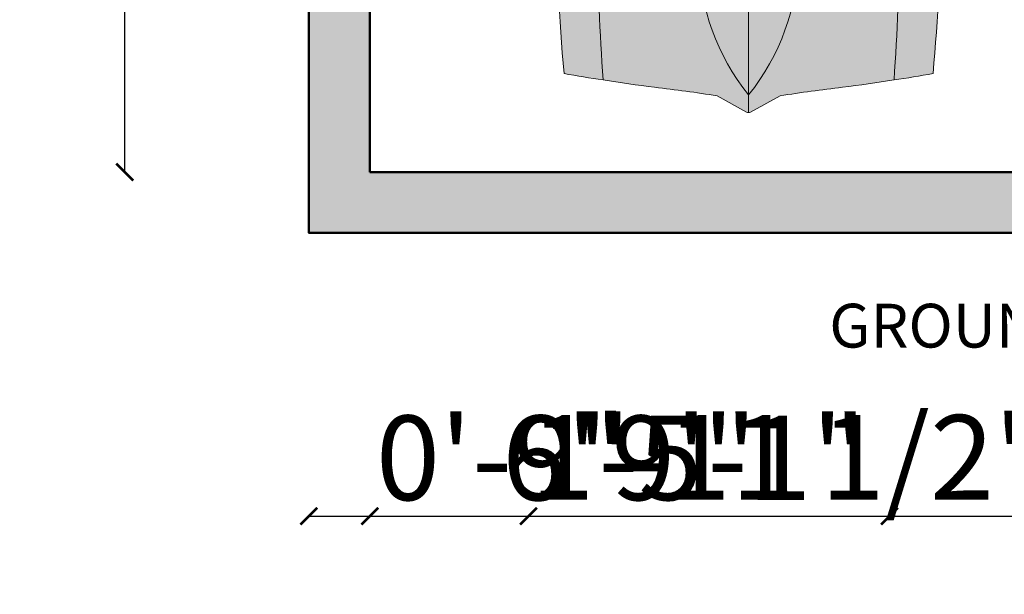
# Model space of a CAD drawing. Units: inches. Extents: x 2419 to 2878, y 1068 to 1713.
# Tile 1 of 20: x 2429 to 2574, y 1068 to 1153. Entities that reach past the tile are written whole.
import ezdxf

# ---------------------------------------------------------------- set-up
doc = ezdxf.new("R2010")
doc.units = ezdxf.units.IN
for name, color, linetype, lineweight in [('A-ANNO-DIMS', 2, 'Continuous', 18), ('A-ANNO-TEXT', 7, 'Continuous', 25), ('A-FLOR-PRKG', 8, 'Continuous', 13), ('A-FLOR-PRKG-PATT', 1, 'Continuous', 13), ('A-WALL', 7, 'Continuous', 50)]:
    doc.layers.add(name, color=color, linetype=linetype, lineweight=lineweight)
doc.layers.add('A-WALL-PATT', color=18, linetype='Continuous', lineweight=13, true_color=0x000000)
doc.styles.get("Standard").update_dxf_attribs({"font": 'arial.ttf'})
doc.dimstyles.new('ISO-25', dxfattribs={"dimtxt": 12.5, "dimasz": 2.5, "dimexe": 1.25, "dimexo": 0.625, "dimtad": 1, "dimdec": 0, "dimlunit": 4, "dimtxsty": 'Standard', "dimblk": 'ARCHTICK', "dimcen": 2.5, "dimse1": 1, "dimse2": 1, "dimclrd": 4, "dimadec": 0, "dimazin": 0, "dimtfac": 1, "dimtdec": 0, "dimtmove": 0, "dimatfit": 3, "dimfxl": 1, "dimarcsym": 0})

# ---------------------------------------------------------------- blocks, each defined once
blk = doc.blocks.new('*U7')
for p, q in [((46.55368679439944, 38.88847654282876), (22.35054758993934, 38.88847654282876)), ((136.6978032355602, 38.88847654282876), (160.90094244002, 38.88847654282867)), ((21.10406751471477, 37.40863046792069), (21.10406751471477, 36.83230215753705)), ((47.80016686962392, 37.39011648242055), (47.80016686962392, 37.40863046792069)), ((135.4513231603356, 37.07354110333037), (135.4513231603356, 37.40863046792069)), ((162.1474225152445, 37.40863046792049), (162.1474225152445, 36.77402019194128)), ((87.98532186932616, 31.87120872459877), (74.75900729854769, 35.92175679182955)), ((134.313356548143, 35.6043097713567), (119.2882629232503, 31.77757799177584)), ((186.4728846989705, -33.49860931502491), (186.4728846989718, 33.49860931502465)), ((188.3990091454065, -32.75868627757393), (188.3990091454077, 32.75868627757058)), ((70.0302824853563, 31.53613089391356), (86.40615155322342, 29.35124891408057)), ((138.4228833961707, 29.35124891408074), (157.2465674415997, 29.35124891408074)), ((186.4728846989718, 29.35124891408083), (167.0083537481071, 29.35124891408083)), ((164.515393597658, 26.39155676426461), (164.5153935976578, -26.39155676426503)), ((32.26591480791686, 11.62530558863241), (36.12873726252356, 17.16961494239206)), ((36.12873726252356, 17.16961494239206), (50.93891189819171, 17.16961494239206)), ((32.12291633764599, 9.505833383620029), (32.12291633764599, 11.15369945057711)), ((58.9167604809788, -10.77488335095668), (58.9167604809788, 10.77488335095617)), ((66.55009204259746, -10.5288681329018), (66.55009204259746, 10.52886813290129)), ((186.4728846989718, -10.5288681329018), (186.4728846989718, 10.52886813290129)), ((29.77279020470884, 9.505833383620029), (51.68362801571248, 9.505833383620029)), ((82.73706193978568, 8.496039918672748), (82.73706193978568, -8.49603991867258)), ((3.266462181856987, 6.128290093440767), (0.1022408397004821, 0.4060708604429806)), ((-4.43e-14, -2.558e-13), (51.68362801571248, -2.558e-13)), ((0.1022408397004821, -0.4060708604432933), (3.266462181856987, -6.128290093441194)), ((29.77279020470884, -9.50583338362054), (51.68362801571248, -9.50583338362054)), ((32.12291633764599, -9.50583338362054), (32.12291633764599, -11.15369945057762)), ((32.26591480791686, -11.62530558863292), (36.12873726252356, -17.16961494239257)), ((36.12873726252356, -17.16961494239257), (50.93891189819171, -17.16961494239257)), ((86.40615155322318, -29.35124891408145), (70.03028248535594, -31.53613089391442)), ((157.2465674415997, -29.35124891408117), (138.4228833961707, -29.35124891408126)), ((167.008353748107, -29.35124891408126), (186.4728846989707, -29.35124891408108)), ((87.98532186932607, -31.87120872459903), (74.7590072985476, -35.92175679182964)), ((134.3133565481428, -35.60430977135721), (119.2882629232503, -31.77757799177618)), ((21.10406751471477, -37.4086304679212), (21.10406751471477, -36.83230215753756)), ((47.80016686962392, -37.39011648242107), (47.80016686962392, -37.4086304679212)), ((135.4513231603355, -37.07354110333088), (135.4513231603355, -37.4086304679212)), ((162.1474225152445, -37.408630467921), (162.1474225152445, -36.77402019194179)), ((46.55368679439944, -38.88847654282927), (22.35054758993934, -38.88847654282927)), ((136.6978032355602, -38.88847654282927), (160.9009424400199, -38.88847654282918))]:
    blk.add_line(p, q)
for centre, major_axis, ratio, start_param, end_param in [((22.35054758993934, 37.40863046792072), (2.08e-14, -1.479846074908118), 0.842303869543976, 3.141592653589776, 4.712388980384677), ((46.55368679439944, 37.40863046792072), (2.2e-14, 1.479846074908118), 0.8423038695439758, -1.570796326794884, 1.73e-14), ((136.6978032355602, 37.40863046792072), (2.357e-13, -1.479846074908118), 0.842303869543976, 3.141592653589603, 4.712388980384554), ((160.90094244002, 37.40863046792052), (5.59e-14, 1.479846074908118), 0.842303869543976, -1.570796326794865, 4.44e-14), ((41.19115208863305, -490.8631038926156), (1.294e-13, 528.2339998381949), 0.8423038695439741, 0.0028100083536837, 0.0755983031096952), ((64.48199294511879, -10555.61767587835), (1.907644e-10, 10593.02630634627), 0.842303869543847, -0.0133969486112073, 0.0027970409639888), ((180.6280394947615, 35.8381667808375), (7.4e-14, 2.219769112362114), 0.8423038695439693, -0.0130174256259048, 1.249894140392862), ((64.48199294754608, -10556.35759891604), (1.349839377e-06, 10595.3130398087), 0.8423038681351469, -0.0133969484821159, -0.0130174254969711), ((183.9799245485226, 33.49860931502124), (3e-16, -2.959692149816168), 0.8423038695439952, 1.570796326796048, 3.128195704978389), ((183.9799245485216, 32.75868627756583), (8.56e-14, -5.246425615115243), 0.8423038695439737, 1.570796326795794, 3.128195704978164), ((266.0300214172791, -27.52442688366631), (1.966072e-10, 313.3077612809058), 0.8423038695435284, 1.367075990158062, 1.391760499156098), ((64.4819929449925, -10555.61767590795), (1.9177683e-09, -10591.54646030096), 0.8423038695482963, 3.133765086725325, 3.140440689641252), ((135.2911776514449, 5.387441675478555), (2.2715e-12, 81.77258453065997), 0.8423038695439563, 1.245306111696802, 1.507880129813836), ((95.78879860270445, -3666.353346297651), (1.949864e-10, -3698.236159209632), 0.8423038695446962, 3.134048706297306, 3.14409775411291), ((37.47375371777758, -593.9621830607928), (6.21e-14, -623.32820996736), 0.8423038695439826, 3.09604606856106, 3.200911180495224), ((134.4003789125686, 5.387441675477674), (4.276e-13, -89.7774543484738), 0.84230386954398, 4.44948196380473, 4.652344057257214), ((149.595361812917, 2.799442537139299), (8.561e-13, -79.57966406425402), 0.842303869543983, 4.372215489277867, 4.640744122441986), ((17.08207736189386, -1.421e-13), (6.87e-14, 147.0179238898305), 0.8423038695439764, 4.511394369635731, 4.913383591133647), ((35.90576140732288, -1.421e-13), (6.87e-14, 147.0179238898305), 0.8423038695439764, 4.511394369635731, 4.913383591133647), ((167.0083537481071, 26.39155676426464), (1.394e-13, 2.959692149816236), 0.842303869543976, 5.55e-14, 1.57079632679492), ((259.1750197310735, -27.52442688366614), (1.506617e-10, -305.3028914627677), 0.8423038695443789, 4.528606069860317, 4.561837674556238), ((-204.4946649195746, 52.39684969293512), (4.12053e-11, -250.9602162198571), 0.8423038695441164, 1.385369446298923, 1.434372047871027), ((13.03653510440275, 17.00972444508943), (1.2303e-12, 27.41599049210566), 0.8423038695439277, 4.435146050259648, 4.718221029521873), ((14.20086229321332, 17.00972444508943), (1.2303e-12, 27.41599049210566), 0.8423038695439277, 4.435146050259648, 4.718221029521873), ((50.7902773840875, 13.33772416300607), (6.340077547122382, -0.356608581037027), 0.6038335755719145, -1.39555193967809, 1.581314658479915), ((32.74615637525823, 11.15369945057713), (1.313e-13, 0.7399230374541176), 0.8423038695439091, 0.8797135699495516, 1.570796326795045), ((29.77279020470884, -46.66302566589627), (5.12e-14, 56.16885904951626), 0.842303869543976, 7e-16, 0.5903187773915901), ((0.6232400376122422, -1.421e-13), (1e-16, -0.7399230374541245), 0.842303869543842, 4.131459131953847, 5.293318828815531), ((29.77279020470884, 46.66302566589578), (4.004e-13, 56.16885904951626), 0.8423038695439734, 2.55127387619821, 3.141592653589801), ((-204.4946649195746, -52.39684969293552), (4.02945e-11, 250.9602162198562), 0.8423038695441192, -1.43437204787103, -1.385369446298926), ((13.03653510440275, -17.00972444508983), (1.2568e-12, -27.41599049210552), 0.8423038695439318, 1.564964277657711, 1.848039256919935), ((14.20086229321332, -17.00972444508983), (1.2568e-12, -27.41599049210552), 0.8423038695439318, 1.564964277657711, 1.848039256919935), ((149.5953618129329, -2.799442537137565), (4.0897e-12, -79.57966406427697), 0.8423038695439419, -1.499151468852248, -1.230622835688196), ((32.74615637525823, -11.1536994505777), (1.3e-13, -0.7399230374541176), 0.8423038695439093, 4.712388980384541, 5.403471737230034), ((134.4003789125684, -5.387441675478584), (4.2949e-12, -89.77745434847827), 0.8423038695439354, -1.510751403667474, -1.307889310215002), ((135.2911776514465, -5.387441675480715), (3.2038e-12, -81.77258453066244), 0.8423038695439492, -1.50788012981387, -1.245306111696839), ((259.1750197310694, 27.52442688365929), (1.08535e-11, 305.3028914629043), 0.8423038695439974, 1.721347632622872, 1.754579237318777), ((167.008353748107, -26.39155676426503), (1.02e-14, -2.959692149816192), 0.8423038695439885, 4.712388980384686, 6.283185307179581), ((266.0300214172791, 27.52442688366566), (8.75241e-11, 313.3077612806533), 0.8423038695441819, 1.749832154434603, 1.774516663432659), ((37.47375371777847, 593.9621830607904), (1.1693e-12, -623.3282099673584), 0.8423038695439528, -0.0593185269054384, 0.0455465850287298), ((95.78879860271888, 3666.35334629765), (1.637818e-10, -3698.236159209629), 0.8423038695447546, -0.0025051005232382, 0.007543947292366), ((183.9799245485216, -33.4986093150211), (9.3e-15, 2.959692149816141), 0.8423038695439732, 3.154989602201626, 4.71238898038339), ((183.9799245485177, -32.7586862775633), (2.428e-13, -5.246425615118353), 0.8423038695439808, 0.0133969486110846, 1.570796326792831), ((41.19115208863322, 490.8631038926152), (1.37757e-11, -528.2339998381949), 0.8423038695440652, -0.0755983031097181, -0.0028100083537155), ((64.48199294503607, 10555.61767590793), (1.6049794e-09, -10591.54646030094), 0.8423038695397146, 0.0011519639481523, 0.0078275668641468), ((22.35054758993934, -37.40863046792117), (2.2e-14, 1.479846074908118), 0.8423038695439758, 1.570796326794908, 3.14159265358981), ((64.48199294495228, 10555.61767590795), (6.117947e-10, 10593.02630637587), 0.8423038695458146, 3.138795612625926, 3.154989602201039), ((46.55368679439944, -37.40863046792117), (2.08e-14, -1.479846074908118), 0.842303869543976, -1.69e-14, 1.570796326794884), ((136.6978032355602, -37.40863046792109), (1.56e-14, -1.479846074908162), 0.8423038695440105, -1.570796326794875, -1.27e-14), ((160.9009424400199, -37.408630467921), (1.969e-13, 1.479846074908162), 0.8423038695440109, 3.141592653589951, 4.712388980384771), ((180.6280394947581, -35.83816678083949), (2.274e-13, -2.219769112363032), 0.8423038695439803, -1.249894138785958, 0.0130174256254374), ((64.48199294197605, 10556.3575989598), (9.365289701e-07, 10595.31303985772), 0.8423038705260315, 3.154610079306566, 3.154989602290631)]:
    blk.add_ellipse(centre, major_axis=major_axis, ratio=ratio, start_param=start_param, end_param=end_param)
at = {"extrusion": (0, 0, -1)}
blk.add_ellipse((50.7902773840875, -13.33772416300655), major_axis=(6.340077547122382, 0.3566085810370246), ratio=0.6038335755719145, start_param=-1.39555193967809, end_param=1.581314658479915, dxfattribs=at)
blk = doc.blocks.new('_ArchTick')
at = {"color": 0, "linetype": 'ByBlock', "const_width": 0.15}
blk.add_lwpolyline([(-0.5, -0.5), (0.5, 0.5)], dxfattribs=at)
blk = doc.blocks.new('*D38')
at = {"layer": 'A-ANNO-DIMS', "color": 4, "lineweight": -2, "transparency": 16777216}
for p, q in [((2444.314464000002, 1165.602617), (2444.314464000002, 1212.505754789905)), ((2444.314464000002, 1130.812987), (2444.314464000002, 1165.602617))]:
    blk.add_line(p, q, dxfattribs=at)
at = {"layer": 'Defpoints', "color": 0, "transparency": 16777216}
for p in [(2444.314464000002, 1165.602617), (2656.740829000001, 1165.602617), (2656.740829000001, 1130.812987)]:
    blk.add_point(p, dxfattribs=at)
at = {"layer": 'A-ANNO-DIMS', "color": 4, "lineweight": -2, "transparency": 16777216, "xscale": 2.5, "yscale": 2.5, "zscale": 2.5}
for p, rotation in [((2444.314464000002, 1165.602617), 90), ((2444.314464000002, 1130.812987), 270)]:
    blk.add_blockref('_ArchTick', p, dxfattribs=dict(at, rotation=rotation))
at = {"layer": 'A-ANNO-DIMS', "color": 0, "transparency": 16777216, "insert": (2437.413884190998, 1190.304185894951), "char_height": 12.5, "attachment_point": 5, "rotation": 90}
blk.add_mtext('2\'-11"', dxfattribs=at)
blk = doc.blocks.new('*D41')
at = {"layer": 'A-ANNO-DIMS', "color": 4, "lineweight": -2, "transparency": 16777216}
for p, q in [((2471.514464, 1079.924615), (2480.514464, 1079.924615)), ((2480.514464, 1079.924615), (2517.492635896316, 1079.924615))]:
    blk.add_line(p, q, dxfattribs=at)
at = {"layer": 'Defpoints', "color": 0, "transparency": 16777216}
for p in [(2480.514464, 1130.812987), (2471.514464, 1121.812987), (2480.514464, 1079.924615)]:
    blk.add_point(p, dxfattribs=at)
at = {"layer": 'A-ANNO-DIMS', "color": 4, "lineweight": -2, "transparency": 16777216, "xscale": 2.5, "yscale": 2.5, "zscale": 2.5, "rotation": 180}
blk.add_blockref('_ArchTick', (2471.514464, 1079.924615), dxfattribs=at)
at = {"layer": 'A-ANNO-DIMS', "color": 4, "lineweight": -2, "transparency": 16777216, "xscale": 2.5, "yscale": 2.5, "zscale": 2.5}
blk.add_blockref('_ArchTick', (2480.514464, 1079.924615), dxfattribs=at)
at = {"layer": 'A-ANNO-DIMS', "color": 0, "transparency": 16777216, "insert": (2500.253549948158, 1086.931777346521), "char_height": 12.5, "attachment_point": 5}
blk.add_mtext('0\'-9"', dxfattribs=at)
blk = doc.blocks.new('*D43')
at = {"layer": 'A-ANNO-DIMS', "color": 4, "lineweight": -2, "transparency": 16777216}
blk.add_line((2480.514464, 1079.924615), (2557.299401, 1079.924615), dxfattribs=at)
at = {"layer": 'Defpoints', "color": 0, "transparency": 16777216}
for p in [(2480.514464, 1408.812987), (2557.299401, 1408.812987), (2557.299401, 1079.924615)]:
    blk.add_point(p, dxfattribs=at)
at = {"layer": 'A-ANNO-DIMS', "color": 4, "lineweight": -2, "transparency": 16777216, "xscale": 2.5, "yscale": 2.5, "zscale": 2.5, "rotation": 180}
blk.add_blockref('_ArchTick', (2480.514464, 1079.924615), dxfattribs=at)
at = {"layer": 'A-ANNO-DIMS', "color": 4, "lineweight": -2, "transparency": 16777216, "xscale": 2.5, "yscale": 2.5, "zscale": 2.5}
blk.add_blockref('_ArchTick', (2557.299401, 1079.924615), dxfattribs=at)
at = {"layer": 'A-ANNO-DIMS', "color": 0, "transparency": 16777216, "insert": (2518.9069325, 1086.931777346521), "char_height": 12.5, "attachment_point": 5}
blk.add_mtext('6\'-5"', dxfattribs=at)
blk = doc.blocks.new('*D44')
at = {"layer": 'A-ANNO-DIMS', "color": 4, "lineweight": -2, "transparency": 16777216}
for p, q in [((2557.299401, 1079.924615), (2585.817994, 1079.924615)), ((2585.817994, 1079.924615), (2652.136206824011, 1079.924615))]:
    blk.add_line(p, q, dxfattribs=at)
at = {"layer": 'Defpoints', "color": 0, "transparency": 16777216}
for p in [(2557.299401, 1408.812987), (2585.817994, 1408.812987), (2585.817994, 1079.924615)]:
    blk.add_point(p, dxfattribs=at)
at = {"layer": 'A-ANNO-DIMS', "color": 4, "lineweight": -2, "transparency": 16777216, "xscale": 2.5, "yscale": 2.5, "zscale": 2.5, "rotation": 180}
blk.add_blockref('_ArchTick', (2557.299401, 1079.924615), dxfattribs=at)
at = {"layer": 'A-ANNO-DIMS', "color": 4, "lineweight": -2, "transparency": 16777216, "xscale": 2.5, "yscale": 2.5, "zscale": 2.5}
blk.add_blockref('_ArchTick', (2585.817994, 1079.924615), dxfattribs=at)
at = {"layer": 'A-ANNO-DIMS', "color": 0, "transparency": 16777216, "insert": (2620.227100412006, 1087.012780075034), "char_height": 12.5, "attachment_point": 5}
blk.add_mtext('2\'-4 1/2"', dxfattribs=at)
blk = doc.blocks.new('*D54')
at = {"layer": 'A-ANNO-DIMS', "color": 4, "lineweight": -2, "transparency": 16777216}
blk.add_line((2444.314464000002, 1130.812987), (2444.314464000002, 1293.812987), dxfattribs=at)
at = {"layer": 'Defpoints', "color": 0, "transparency": 16777216}
for p in [(2444.314464000002, 1293.812987), (2480.514464000001, 1293.812987), (2480.514464000001, 1130.812987)]:
    blk.add_point(p, dxfattribs=at)
at = {"layer": 'A-ANNO-DIMS', "color": 4, "lineweight": -2, "transparency": 16777216, "xscale": 2.5, "yscale": 2.5, "zscale": 2.5}
for p, rotation in [((2444.314464000002, 1293.812987), 90), ((2444.314464000002, 1130.812987), 270)]:
    blk.add_blockref('_ArchTick', p, dxfattribs=dict(at, rotation=rotation))
at = {"layer": 'A-ANNO-DIMS', "color": 0, "transparency": 16777216, "insert": (2437.30303835198, 1212.312987), "char_height": 12.5, "attachment_point": 5, "rotation": 90}
blk.add_mtext('13\'-7"', dxfattribs=at)
blk = doc.blocks.new('*D56')
at = {"layer": 'A-ANNO-DIMS', "color": 4, "lineweight": -2, "transparency": 16777216}
for p, q in [((2480.514464, 1079.924615), (2503.967101000001, 1079.924615)), ((2503.967101000001, 1079.924615), (2578.607278353343, 1079.924615))]:
    blk.add_line(p, q, dxfattribs=at)
at = {"layer": 'Defpoints', "color": 0, "transparency": 16777216}
for p in [(2480.514464, 1507.812987), (2503.967101000001, 1494.852151), (2503.967101000001, 1079.924615)]:
    blk.add_point(p, dxfattribs=at)
at = {"layer": 'A-ANNO-DIMS', "color": 4, "lineweight": -2, "transparency": 16777216, "xscale": 2.5, "yscale": 2.5, "zscale": 2.5, "rotation": 180}
blk.add_blockref('_ArchTick', (2480.514464, 1079.924615), dxfattribs=at)
at = {"layer": 'A-ANNO-DIMS', "color": 4, "lineweight": -2, "transparency": 16777216, "xscale": 2.5, "yscale": 2.5, "zscale": 2.5}
blk.add_blockref('_ArchTick', (2503.967101000001, 1079.924615), dxfattribs=at)
at = {"layer": 'A-ANNO-DIMS', "color": 0, "transparency": 16777216, "insert": (2542.537189676672, 1087.012780075034), "char_height": 12.5, "attachment_point": 5}
blk.add_mtext('1\'-11 1/2"', dxfattribs=at)
blk = doc.blocks.new('*D59')
at = {"layer": 'A-ANNO-DIMS', "color": 4, "lineweight": -2, "transparency": 16777216}
blk.add_line((2480.514464, 1079.924615), (2589.514464, 1079.924615), dxfattribs=at)
at = {"layer": 'Defpoints', "color": 0, "transparency": 16777216}
for p in [(2480.514464, 1414.812987), (2589.514464, 1414.812987), (2589.514464, 1079.924615)]:
    blk.add_point(p, dxfattribs=at)
at = {"layer": 'A-ANNO-DIMS', "color": 4, "lineweight": -2, "transparency": 16777216, "xscale": 2.5, "yscale": 2.5, "zscale": 2.5, "rotation": 180}
blk.add_blockref('_ArchTick', (2480.514464, 1079.924615), dxfattribs=at)
at = {"layer": 'A-ANNO-DIMS', "color": 4, "lineweight": -2, "transparency": 16777216, "xscale": 2.5, "yscale": 2.5, "zscale": 2.5}
blk.add_blockref('_ArchTick', (2589.514464, 1079.924615), dxfattribs=at)
at = {"layer": 'A-ANNO-DIMS', "color": 0, "transparency": 16777216, "insert": (2535.014464, 1086.931777346521), "char_height": 12.5, "attachment_point": 5}
blk.add_mtext('9\'-1"', dxfattribs=at)

msp = doc.modelspace()

# ---------------------------------------------------------------- hatches: boundary and pattern name
at = {"layer": 'A-FLOR-PRKG-PATT'}
h = msp.add_hatch(color=256, dxfattribs=at)
h.dxf.hatch_style = 1
edge = h.paths.add_edge_path(flags=17)
edge.add_line((2558.78367155362, 1281.34848374267), (2514.160945116646, 1281.348483742671))
edge.add_line((2514.160945116646, 1281.348483742671), (2514.160945116646, 1266.552513009246))
edge.add_ellipse((2516.410756249479, 1266.552513009246), major_axis=(2.249811132832746, 7.445e-13), ratio=0.8423038695441503, start_angle=179.999999999981, end_angle=269.999999999981)
edge.add_line((2516.410756249479, 1264.657488386317), (2556.533860420787, 1264.657488386317))
edge.add_ellipse((2556.533860420787, 1266.552513009246), major_axis=(2.249811132833201, 8.993e-13), ratio=0.8423038695438791, start_angle=269.9999999999771, end_angle=359.9999999999771)
edge.add_line((2558.78367155362, 1266.552513009246), (2558.78367155362, 1281.34848374267))
edge = h.paths.add_edge_path()
edge.add_ellipse((-5487.384552136685, 1188.617060175704), major_axis=(8052.293045395979, 3.62524e-11), ratio=0.8423038695435844, start_angle=0.3838667787920817, end_angle=0.5282714718171219)
edge.add_ellipse((-5487.384552136685, 1188.617060175704), major_axis=(8052.293045395979, 3.62524e-11), ratio=0.8423038695435844, start_angle=0.5282714718171219, end_angle=0.6465540970607009)
edge.add_ellipse((2561.936289167072, 1279.453459119742), major_axis=(-2.249811132833226, 1.1022e-12), ratio=0.8423038695438698, start_angle=180.6465540971199, end_angle=269.9999999999318)
edge.add_line((2561.936289167075, 1281.34848374267), (2558.78367155362, 1281.34848374267))
edge.add_line((2558.78367155362, 1281.34848374267), (2558.78367155362, 1266.266612494733))
edge.add_ellipse((2556.533860420787, 1266.552513009246), major_axis=(2.249811132833201, 8.993e-13), ratio=0.8423038695438791, start_angle=269.9999999999771, end_angle=359.9999999999771, ccw=False)
edge.add_line((2556.533860420787, 1264.657488386317), (2516.071329440636, 1264.657488386317))
edge.add_ellipse((2516.410756249479, 1266.552513009246), major_axis=(2.249811132832746, 7.445e-13), ratio=0.8423038695441503, start_angle=179.9999999999811, end_angle=269.999999999981, ccw=False)
edge.add_line((2514.160945116646, 1266.552513009246), (2514.160945116646, 1281.348483742671))
edge.add_line((2514.160945116646, 1281.348483742671), (2511.008327503191, 1281.348483742671))
edge.add_ellipse((2511.008327503194, 1279.453459119743), major_axis=(2.249811132832755, 8.714e-13), ratio=0.842303869544046, start_angle=90.00000000004655, end_angle=179.3534459029089)
edge.add_ellipse((10560.32916878445, 1188.617060175834), major_axis=(8052.293045373481, 7.264082e-10), ratio=0.842303869546111, start_angle=179.3534459029329, end_angle=179.3813568036756)
edge.add_ellipse((10560.32916878445, 1188.617060175834), major_axis=(8052.293045373481, 7.264082e-10), ratio=0.842303869546111, start_angle=179.3813568036756, end_angle=179.4717285281769)
edge.add_ellipse((10560.32916878445, 1188.617060175834), major_axis=(8052.293045373481, 7.264082e-10), ratio=0.842303869546111, start_angle=179.4717285281769, end_angle=179.6161332212023)
edge.add_ellipse((10560.32916878445, 1188.617060175834), major_axis=(8052.293045373481, 7.264082e-10), ratio=0.842303869546111, start_angle=179.6161332212023, end_angle=180.0902290885891)
edge.add_ellipse((10560.32916878445, 1188.617060175834), major_axis=(8052.293045373481, 7.264082e-10), ratio=0.842303869546111, start_angle=180.0902290885891, end_angle=180.1349865768531)
edge.add_ellipse((2909.602086681569, 1170.912518487192), major_axis=(401.537279358841, 1.00104e-11), ratio=0.8423038695439784, start_angle=180.1806905311021, end_angle=182.1799503136438)
edge.add_ellipse((2909.602086681569, 1170.912518487192), major_axis=(401.537279358841, 1.00104e-11), ratio=0.8423038695439784, start_angle=182.1799503136438, end_angle=183.6504275856975)
edge.add_ellipse((2557.395012080375, 1341.823872000969), major_axis=(238.1610159604077, 8.386761e-10), ratio=0.8423038695464203, start_angle=256.2194710103002, end_angle=257.874034447514)
edge.add_ellipse((2987.972891601874, 1168.086736677267), major_axis=(-473.8231799819343, 8.8666e-12), ratio=0.8423038695441055, start_angle=-2.19854056595409, end_angle=2.8637146078386877, ccw=False)
edge.add_ellipse((2532.377042461035, 1241.765548321486), major_axis=(-68.24436665927666, 5.9291e-12), ratio=0.8423038695438547, start_angle=72.28004677725448, end_angle=85.9175893088543)
edge.add_line((2528.281776586936, 1184.386646564943), (2544.66284008333, 1184.386646564943))
edge.add_ellipse((2540.567574209232, 1241.765548321486), major_axis=(68.24436665927627, 7.0353e-12), ratio=0.8423038695438563, start_angle=-85.91758930885564, end_angle=-72.28004677725573)
edge.add_ellipse((2084.971725068394, 1168.086736677268), major_axis=(473.8231799819329, 7.7093e-12), ratio=0.842303869544119, start_angle=-2.863714607838574, end_angle=2.19854056595409, ccw=False)
edge.add_ellipse((2515.549604589891, 1341.823872000969), major_axis=(238.1610159617672, 7.268827e-10), ratio=0.8423038695418011, start_angle=-77.87403444789076, end_angle=-76.21947101067707)
edge.add_ellipse((2163.342529988697, 1170.912518487192), major_axis=(401.5372793588411, 5.38767e-11), ratio=0.8423038695443597, start_angle=-3.650427585706752, end_angle=-2.179950313652928)
edge.add_ellipse((2163.342529988697, 1170.912518487192), major_axis=(401.5372793588411, 5.38767e-11), ratio=0.8423038695443597, start_angle=-2.179950313652928, end_angle=-0.1356123904461693)
edge.add_ellipse((-5487.384552136685, 1188.617060175704), major_axis=(8052.293045395979, 3.62524e-11), ratio=0.8423038695435844, start_angle=-0.1349865768572857, end_angle=-0.0902290885934275)
edge.add_ellipse((-5487.384552136685, 1188.617060175704), major_axis=(8052.293045395979, 3.62524e-11), ratio=0.8423038695435844, start_angle=-0.0902290885934275, end_angle=0.3838667787920817)
edge = h.paths.add_edge_path(flags=16)
edge.add_ellipse((2538.600305662885, 1253.316020452369), major_axis=(-60.4925124290502, 2.2066e-12), ratio=0.8423038695439758, start_angle=94.87006959713776, end_angle=112.7919148775885)
edge.add_line((2558.78367155362, 1205.282717824576), (2560.444510435955, 1192.834594616562))
edge.add_ellipse((2540.567574209233, 1242.442689327507), major_axis=(62.15946177006578, 2.00584e-11), ratio=0.8423038695437449, start_angle=-85.72257903696442, end_angle=-68.16504620330988, ccw=False)
edge.add_line((2544.475831520138, 1190.18912650496), (2528.468785150127, 1190.18912650496))
edge.add_ellipse((2532.377042461034, 1242.442689327506), major_axis=(-62.15946177005032, 4.9036e-12), ratio=0.8423038695439334, start_angle=68.16504620329499, end_angle=85.72257903694901, ccw=False)
edge.add_line((2512.500106234312, 1192.834594616562), (2514.160945116646, 1205.282717824576))
edge.add_ellipse((2534.344311007379, 1253.316020452358), major_axis=(60.49251242903284, 5.7929e-12), ratio=0.8423038695440167, start_angle=247.2080851224046, end_angle=265.1299304028586)
edge.add_line((2530.014040303706, 1202.493657935295), (2542.93057636656, 1202.493657935295))
edge = h.paths.add_edge_path(flags=16)
edge.add_ellipse((-250.5076064213731, 1212.41494060954), major_axis=(2811.215647327496, 7.69506e-11), ratio=0.8423038695473968, start_angle=-0.1208973690345315, end_angle=0.3640763488885457)
edge.add_line((2560.628046540813, 1230.278067505092), (2563.536938183683, 1241.699398237495))
edge.add_ellipse((-5487.384552136674, 1188.617060175768), major_axis=(8051.168139829552, 1.0212802e-09), ratio=0.8423038695408568, start_angle=0.05559431349178112, end_angle=0.3777641939024079, ccw=False)
edge.add_line((2563.77824565912, 1196.42913661293), (2560.699219978594, 1206.483124751376))
edge = h.paths.add_edge_path(flags=16)
edge.add_ellipse((2536.472308335133, 1152.58599600549), major_axis=(111.7557317283417, 6.024e-13), ratio=0.8423038695439972, start_angle=76.40186530976897, end_angle=103.5981346902301)
edge.add_line((2514.160945116646, 1244.823256661064), (2514.160945116646, 1259.132087371369))
edge.add_ellipse((2536.472308335133, 1166.894826715795), major_axis=(111.7557317283482, 6.52e-13), ratio=0.8423038695439483, start_angle=76.401865309769, end_angle=103.5981346902301, ccw=False)
edge.add_line((2558.78367155362, 1259.13208737137), (2558.78367155362, 1244.823256661064))
edge = h.paths.add_edge_path(flags=16)
edge.add_line((2512.24539669167, 1206.483124751367), (2509.166371011145, 1196.429136612926))
edge.add_ellipse((10560.32916880695, 1188.617060175738), major_axis=(8051.168139829567, 3.955788e-10), ratio=0.8423038695452166, start_angle=179.6222358060874, end_angle=179.9444056864979, ccw=False)
edge.add_line((2509.407678486582, 1241.699398237499), (2512.316570129453, 1230.278067505094))
edge.add_ellipse((5323.452223091639, 1212.41494060953), major_axis=(2811.215647327498, 3.441147e-10), ratio=0.8423038695471676, start_angle=179.6359236511027, end_angle=180.1208973690256)
edge = h.paths.add_edge_path()
edge.add_ellipse((2084.971725068394, 1168.086736677268), major_axis=(473.8231799819329, 7.7093e-12), ratio=0.842303869544119, start_angle=-2.863714607838618, end_angle=2.198540565954143)
edge.add_ellipse((2540.567574209232, 1241.765548321486), major_axis=(68.24436665927627, 7.0353e-12), ratio=0.8423038695438563, start_angle=-85.91758930885561, end_angle=-72.28004677725562, ccw=False)
edge.add_line((2544.66284008333, 1184.386646564943), (2528.281776586936, 1184.386646564943))
edge.add_ellipse((2532.377042461035, 1241.765548321486), major_axis=(-68.24436665927666, 5.9291e-12), ratio=0.8423038695438547, start_angle=72.28004677725448, end_angle=85.91758930885442, ccw=False)
edge.add_ellipse((2987.972891601874, 1168.086736677267), major_axis=(-473.8231799819343, 8.8666e-12), ratio=0.8423038695441055, start_angle=-2.198540565954097, end_angle=2.86371460783868)
edge.add_ellipse((2557.395012080375, 1336.613039816894), major_axis=(232.0761110713879, 4.935805e-10), ratio=0.8423038695458167, start_angle=257.5553727064329, end_angle=259.7904610027336)
edge.add_ellipse((2496.642822767904, 984.1543496287911), major_axis=(190.7675054597987, 1.126016e-10), ratio=0.8423038695444711, start_angle=77.44506735582888, end_angle=80.7434339927645, ccw=False)
edge.add_line((2531.813886249475, 1142.084050780911), (2536.163633413452, 1139.678766703385))
edge.add_ellipse((2536.472308335133, 1140.07480444526), major_axis=(-0.5624527832082081, 2e-16), ratio=0.8423038695442194, start_angle=52.06686954015882, end_angle=90.00000000000001)
edge.add_line((2536.472308335133, 1139.601048289528), (2536.472308335133, 1142.214540749464))
edge.add_ellipse((2571.943225349704, 1162.232846283187), major_axis=(42.69677993908317, 2.1357e-12), ratio=0.8423038695439387, start_angle=179.9999999999972, end_angle=209.4385695979767, ccw=False)
edge.add_line((2529.246445410621, 1162.232846283187), (2529.246445410621, 1164.019295572439))
edge.add_line((2529.246445410621, 1164.019295572439), (2527.791345403533, 1164.019295572439))
edge.add_line((2527.791345403533, 1164.019295572439), (2523.420818893486, 1167.064321898398))
edge.add_line((2523.420818893486, 1167.064321898398), (2523.420818893486, 1178.322281877985))
edge.add_ellipse((2526.333632152054, 1178.20929729458), major_axis=(0.2710761508483066, 4.819412400518167), ratio=0.6038335755720334, start_angle=-73.65740804575063, end_angle=90.99798572492182, ccw=False)
edge.add_line((2529.246445410621, 1178.88837812286), (2529.246445410621, 1162.232846283187))
edge.add_ellipse((2571.943225349704, 1162.232846283187), major_axis=(42.69677993908317, 2.1357e-12), ratio=0.8423038695439387, start_angle=179.9999999999971, end_angle=209.4385695979767)
edge.add_ellipse((2501.001391320562, 1162.232846283187), major_axis=(42.69677993908317, 6.184e-12), ratio=0.8423038695440235, start_angle=-29.43856959798787, end_angle=-8.2942e-12)
edge.add_line((2543.698171259645, 1162.232846283187), (2543.698171259645, 1178.88837812286))
edge.add_ellipse((2546.610984518212, 1178.20929729458), major_axis=(-0.2710761508525395, 4.819412400518348), ratio=0.6038335755718809, start_angle=269.00201427502856, end_angle=433.65740804570055, ccw=False)
edge.add_line((2549.52379777678, 1178.322281877985), (2549.52379777678, 1167.064321898398))
edge.add_line((2549.52379777678, 1167.064321898398), (2545.153271266734, 1164.019295572439))
edge.add_line((2545.153271266734, 1164.019295572439), (2543.698171259645, 1164.019295572439))
edge.add_line((2543.698171259645, 1164.019295572439), (2543.698171259645, 1162.232846283187))
edge.add_ellipse((2501.001391320562, 1162.232846283187), major_axis=(42.69677993908317, 6.184e-12), ratio=0.8423038695440235, start_angle=-29.438569597987794, end_angle=-8.29913915367797e-12, ccw=False)
edge.add_line((2536.472308335133, 1142.214540749463), (2536.472308335133, 1139.601048289528))
edge.add_ellipse((2536.472308335133, 1140.07480444526), major_axis=(-0.5624527832082081, 2e-16), ratio=0.8423038695442194, start_angle=90.00000000000001, end_angle=127.9331304598412)
edge.add_line((2536.780983256814, 1139.678766703385), (2541.130730420792, 1142.084050780911))
edge.add_ellipse((2576.301793902363, 984.1543496287911), major_axis=(190.767505459939, 3.39412e-11), ratio=0.8423038695438718, start_angle=99.25656600719128, end_angle=102.55493264412712, ccw=False)
edge.add_ellipse((2515.549604589896, 1336.613039816892), major_axis=(-232.0761110718477, 5.10817e-11), ratio=0.8423038695441782, start_angle=100.2095389971557, end_angle=102.4446272934566)
at = {"layer": 'A-WALL-PATT'}
h = msp.add_hatch(color=256, dxfattribs=at)
h.dxf.hatch_style = 1
h.paths.add_polyline_path([(2780.514463761465, 1577.812987234935), (2471.514463761465, 1577.812987234935), (2471.514463761465, 1121.812987234935), (2780.514463761465, 1121.812987234935)])
h.paths.add_polyline_path([(2480.514463761465, 1568.812987234935), (2771.514463761465, 1568.812987234935), (2771.514463761465, 1130.812987234935), (2480.514463761465, 1130.812987234935)], flags=16)
h.paths.add_polyline_path([(2528.514463761465, 1568.812987234935), (2528.514463761465, 1512.812987234935), (2594.514463761465, 1512.812987234935), (2594.514463761465, 1414.812987234935), (2596.568399739099, 1414.812987234935), (2596.568399739099, 1441.609368546496), (2597.816088158561, 1441.609368546496), (2597.816088158561, 1441.582062289591, -0.38401605427067), (2625.03494332709, 1414.812987234935), (2725.514463761465, 1414.812987234935), (2725.514463761465, 1567.54501314674), (2728.302225194595, 1567.54501314674), (2746.887301415459, 1567.54501314674), (2746.887301415459, 1566.731916062077), (2746.869506397459, 1566.731916062077, -0.3672161804255682), (2730.514463761465, 1549.092071412193), (2730.514463761465, 1512.812987234935), (2750.853045566032, 1512.812987234935), (2750.853045566032, 1510.025225801806, -0.4014527144963593), (2733.081066429831, 1491.457944598941), (2733.081066429831, 1491.440149580942), (2732.267969345168, 1491.440149580942), (2732.267969345168, 1507.812987234935), (2730.514463761465, 1507.812987234935), (2730.514463761465, 1408.812987234935), (2736.514463761465, 1408.812987234935), (2736.514463761466, 1349.812987234935), (2632.514463761465, 1349.812987234935), (2632.514463761465, 1408.812987234935), (2528.514463761465, 1408.812987234935), (2528.514463761465, 1414.812987234935), (2503.967100522841, 1414.812987234935), (2503.967100522841, 1494.852151014206), (2558.37888418044, 1494.852151014206), (2558.37888418044, 1507.812987234935), (2529.964934876797, 1507.812987234936, -0.4142135623730951), (2530.820819834016, 1506.957102277716), (2530.820819834016, 1497.257075044924, -0.4142135623730951), (2529.964934876797, 1496.401190087705), (2514.55900564685, 1496.401190087705, -0.4142135623730903), (2513.703120689631, 1497.257075044924), (2513.703120689631, 1506.957102277716, -0.4142135623730951), (2514.55900564685, 1507.812987234936), (2528.514463761465, 1507.812987234936), (2528.514463761465, 1512.812987234935), (2480.514463761465, 1512.812987234935)], flags=0)
h.paths.add_polyline_path([(2516.261971761824, 1507.812987234935), (2528.261968761824, 1507.812987234935), (2528.261968761824, 1505.812987234935), (2523.416669079506, 1505.812987234935), (2524.073835609436, 1504.674744674158), (2529.394344905318, 1504.674744674158, -0.4142135623730951), (2529.964934876797, 1504.104154702678), (2529.964934876797, 1497.827665016404, -0.4142135623730951), (2529.394344905318, 1497.257075044924), (2515.12959561833, 1497.257075044924, -0.4142135623730987), (2514.55900564685, 1497.827665016404), (2514.55900564685, 1504.104154702678, -0.4142135623730951), (2515.12959561833, 1504.674744674158), (2520.688784298745, 1504.674744674158), (2521.342314766239, 1505.812987234935), (2516.261971761824, 1505.812987234935)], flags=0)
h.paths.add_polyline_path([(2522.015649482737, 1505.530629631377), (2522.816542912466, 1507.317910507759, -0.6550601971121365), (2522.254220692544, 1506.063027257721), (2522.194533044389, 1505.929827773067), (2522.425009080837, 1505.530629631377)], flags=0)
h.paths.add_polyline_path([(2522.832560233303, 1500.965909859541, -1), (2521.691380290344, 1500.965909859541, -1)], flags=0)
h.paths.add_polyline_path([(2522.547265247564, 1500.965909859541, -1), (2521.976675276084, 1500.965909859541, -1)], flags=0)
h.paths.add_polyline_path([(2482.005175746464, 1470.632511127513), (2499.893716585039, 1470.632511127513), (2499.893716585039, 1448.271831352515), (2482.005175746464, 1448.271831352515), (2482.005175746464, 1452.743967307515), (2481.259819753965, 1452.743967307515), (2481.259819753965, 1449.762543337515), (2480.514463761465, 1449.762543337515), (2480.514463761465, 1469.141799142513), (2481.259819753965, 1469.141799142513), (2481.259819753965, 1466.160375172514), (2482.005175746464, 1466.160375172514)], flags=0)
h.paths.add_polyline_path([(2488.71337669754, 1466.160375172514, -1), (2484.24124074254, 1466.160375172514, -1)], flags=0)
h.paths.add_polyline_path([(2496.166936473468, 1466.160375172514, -1), (2490.204088533468, 1466.160375172514, -1)], flags=0)
h.paths.add_polyline_path([(2487.96802070504, 1466.160375172514, -1), (2484.986596735041, 1466.160375172514, -1)], flags=0)
h.paths.add_polyline_path([(2495.421580480968, 1466.160375172514, -1), (2490.949444525969, 1466.160375172514, -1)], flags=0)
h.paths.add_polyline_path([(2487.22266471254, 1466.160375172514, -1), (2485.731952727541, 1466.160375172514, -1)], flags=0)
h.paths.add_polyline_path([(2494.676224488468, 1466.160375172514, -1), (2491.694800518468, 1466.160375172514, -1)], flags=0)
h.paths.add_polyline_path([(2499.10799430668, 1468.004897240262, -1), (2497.977225324558, 1468.004897240262, -1)], flags=0)
h.paths.add_polyline_path([(2493.930868495968, 1466.160375172514, -1), (2492.440156510968, 1466.160375172514, -1)], flags=0)
h.paths.add_polyline_path([(2499.37156767049, 1463.70992381177, -1), (2498.1659645309, 1463.70992381177, -1)], flags=0)
h.paths.add_polyline_path([(2484.241243723964, 1461.688239217514), (2496.16693662254, 1461.688239217514), (2496.16693662254, 1457.216103262515), (2484.241243723964, 1457.216103262515)], flags=0)
h.paths.add_polyline_path([(2484.986599716464, 1460.942883225014), (2495.42158063004, 1460.942883225014), (2495.42158063004, 1457.961459255015), (2484.986599716464, 1457.961459255015)], flags=0)
h.paths.add_polyline_path([(2586.879843577569, 1510.025225801806), (2587.692940662232, 1510.025225801806), (2587.692940662232, 1491.440149580942), (2586.879843577569, 1491.440149580942)], flags=0)
h.paths.add_polyline_path([(2499.258769311151, 1459.414950383278, -1), (2498.203381609636, 1459.414950383278, -1)], flags=0)
h.paths.add_polyline_path([(2489.45873269004, 1452.743967307515, -1), (2483.49588475004, 1452.743967307515, -1)], flags=0)
h.paths.add_polyline_path([(2557.29940140061, 1408.812987234935), (2557.29940140061, 1413.090776101661, -0.4014527144963548), (2584.570305425984, 1441.582062289591), (2584.570305425984, 1441.609368546496), (2585.817993845445, 1441.609368546496), (2585.817993845445, 1413.090776101661), (2585.817993845445, 1408.812987234935)], flags=0)
h.paths.add_polyline_path([(2488.71337669754, 1452.743967307515, -1), (2484.24124074254, 1452.743967307515, -1)], flags=0)
h.paths.add_polyline_path([(2495.421580480968, 1452.743967307515, -1), (2490.949444525969, 1452.743967307515, -1)], flags=0)
h.paths.add_polyline_path([(2487.96802070504, 1452.743967307515, -1), (2484.986596735041, 1452.743967307515, -1)], flags=0)
h.paths.add_polyline_path([(2494.676224488468, 1452.743967307515, -1), (2491.694800518468, 1452.743967307515, -1)], flags=0)
h.paths.add_polyline_path([(2487.22266471254, 1452.743967307515, -1), (2485.731952727541, 1452.743967307515, -1)], flags=0)
h.paths.add_polyline_path([(2499.18308934039, 1454.441826005015, -1), (2497.902130290848, 1454.441826005015, -1)], flags=0)
h.paths.add_polyline_path([(2493.930868495968, 1452.743967307515, -1), (2492.440156510968, 1452.743967307515, -1)], flags=0)
h.paths.add_polyline_path([(2499.296459951454, 1450.636626811365, -1), (2497.788759679783, 1450.636626811365, -1)], flags=0)
h.paths.add_polyline_path([(2619.128766651402, 1558.889032727177, -1), (2605.128766651402, 1558.889032727177, -1)], flags=0)
h.paths.add_polyline_path([(2609.128766651402, 1558.889032727177), (2612.128766651402, 1561.889033727177), (2615.128769651402, 1558.889032727177), (2612.128766651402, 1555.889032727177)], flags=0)
h.paths.add_polyline_path([(2611.128766651402, 1558.889032727177, -1), (2613.128766651402, 1558.889032727177, -1)], flags=0)
h.paths.add_polyline_path([(2633.678910285153, 1568.812987234935), (2693.678900285153, 1568.812987234935), (2693.678900285153, 1488.812957234935), (2633.678910285153, 1488.812957234935)], flags=0)
h.paths.add_polyline_path([(2641.678900285152, 1554.412987234935), (2641.678900285152, 1567.612987234935), (2662.478890285152, 1567.612987234935), (2662.478890285152, 1554.412987234935), (2664.878900285153, 1554.412987234935), (2664.878900285153, 1567.612987234935), (2685.678900285152, 1567.612987234935), (2685.678900285152, 1552.412987234935), (2680.478908969363, 1552.412987234935), (2693.678900285153, 1539.212987234935), (2678.478910285153, 1539.212987234935), (2678.478910285153, 1554.412987234935)], flags=0)
h.paths.add_polyline_path([(2637.514463761465, 1408.812987234935), (2731.514463761465, 1408.812987234935), (2731.514463761465, 1354.812987234935), (2637.514463761465, 1354.812987234935), (2637.514463761465, 1357.97634876414), (2635.302225194595, 1357.97634876414), (2635.302225194595, 1358.789445848803), (2637.514463761465, 1358.789445848803)], flags=0)
h.paths.add_polyline_path([(2717.171392308236, 1559.642859555671, -1), (2703.171392308235, 1559.642859555671, -1)], flags=0)
h.paths.add_polyline_path([(2707.171392308235, 1559.642859555671), (2710.171392308236, 1562.642860555671), (2713.171395308235, 1559.642859555671), (2710.171392308236, 1556.642859555671)], flags=0)
h.paths.add_polyline_path([(2709.171392308235, 1559.642859555671, -1), (2711.171392308235, 1559.642859555671, -1)], flags=0)
h.paths.add_polyline_path([(2685.37839484874, 1408.812987234935), (2706.37839484874, 1408.812987234935), (2706.37839484874, 1400.812987234935), (2699.87839484874, 1400.812987234935), (2701.8783582045, 1394.813097167654, -0.5013234908365424), (2696.923094014159, 1375.951847407521, -0.1328909081880473), (2694.833737505469, 1375.951847423997, -0.5013167773010871), (2689.878359877304, 1394.812882320626), (2691.87839484874, 1400.812987234935), (2688.87839484874, 1400.812987234935), (2688.87839484874, 1399.312987234935), (2685.87839484874, 1399.312987234935), (2685.87839484874, 1400.312987234935), (2687.87839484874, 1400.312987234935), (2687.87839484874, 1400.812987234935), (2685.37839484874, 1400.812987234935)], flags=0)
h.paths.add_polyline_path([(2687.378395015029, 1407.812987234935), (2704.37839468245, 1407.812987234935, -0.5000001164019596), (2705.37839484874, 1406.812987068648), (2705.37839484874, 1402.812987401223, -0.5000001164019594), (2704.37839468245, 1401.812987234935), (2687.378395015029, 1401.812987234935, -0.5000001164019899), (2686.37839484874, 1402.812987401223), (2686.37839484874, 1406.812987068648, -0.5000001164019594)], flags=0)
h.paths.add_polyline_path([(2639.514463761465, 1205.812987234935), (2634.514463761465, 1205.812987234935), (2634.514463761464, 1293.812987234935), (2637.514463761466, 1293.812987234935), (2639.514463761465, 1293.812987234935)], flags=0)
h.paths.add_polyline_path([(2691.878449271624, 1394.812987234935), (2699.878439365793, 1394.812987234935, -0.4800795019661124), (2697.522447975332, 1377.289995604548, -0.2150037826744892), (2694.234383577574, 1377.28999563916, -0.4800796505540576)], flags=0)
h.paths.add_polyline_path([(2757.514358847156, 1453.891486469081), (2763.514463761465, 1451.891451497645), (2763.514463761465, 1454.891451497645), (2762.014463761465, 1454.891451497645), (2762.014463761465, 1457.891451497645), (2763.014463761465, 1457.891451497645), (2763.014463761465, 1455.891451497645), (2763.514463761465, 1455.891451497645), (2763.514463761465, 1458.391451497645), (2771.514463761465, 1458.391451497645), (2771.514463761465, 1437.391451497645), (2763.514463761465, 1437.391451497645), (2763.514463761465, 1443.891451497645), (2757.514573694182, 1441.891488141884, -0.5013234908367097), (2738.653323934048, 1446.846752332236, -0.1328909081861904), (2738.653323950519, 1448.936108840897, -0.5013167773016524)], flags=0)
h.paths.add_polyline_path([(2739.991472165689, 1449.535462768808, -0.4800796505541595), (2757.514463761465, 1451.891397074762), (2757.514463761465, 1443.891406980593, -0.4800795019659427), (2739.991472131081, 1446.247398371048, -0.2150037826747098)], flags=0)
h.paths.add_polyline_path([(2765.514463927754, 1457.391451497645), (2769.514463595176, 1457.391451497645, -0.500000116401859), (2770.514463761465, 1456.391451331358), (2770.514463761465, 1439.391451663933, -0.500000116401859), (2769.514463595176, 1438.391451497645), (2765.514463927754, 1438.391451497645, -0.500000116401859), (2764.514463761465, 1439.391451663933), (2764.514463761465, 1456.391451331358, -0.5000001164020391)], flags=0)

# ---------------------------------------------------------------- linework, layer by layer
at = {"layer": 'A-WALL'}
for p, q in [((2480.514463761465, 1130.812987234935), (2480.514463761465, 1568.812987234935)), ((2771.514463761465, 1130.812987234935), (2480.514463761465, 1130.812987234935))]:
    msp.add_line(p, q, dxfattribs=at)
msp.add_lwpolyline([(2471.514463761465, 1577.812987234935), (2780.514463761465, 1577.812987234935), (2780.514463761465, 1121.812987234935), (2471.514463761465, 1121.812987234935)], close=True, dxfattribs=at)

# ---------------------------------------------------------------- block references
at = {"layer": 'A-FLOR-PRKG', "xscale": 0.7601503869153388, "yscale": 0.7601503869153388, "zscale": 0.7601503869153388, "rotation": 90}
msp.add_blockref('*U7', (2536.472308335133, 1139.601048289528), dxfattribs=at)

# ---------------------------------------------------------------- texts
at = {"layer": 'A-ANNO-TEXT'}
msp.add_text('GROUND FLOOR PLAN', height=6.475338566187019, dxfattribs=at).set_placement((2548.400159616928, 1104.861116923859))

# ---------------------------------------------------------------- dimensions: what is measured, and where the dimension line sits
at = {"layer": 'A-ANNO-DIMS'}
for base, p1, p2, picture, middle in [((2503.967101000001, 1079.924615), (2480.514464, 1507.812987), (2503.967101000001, 1494.852151), '*D56', (2542.537189676672, 1087.012780075034)), ((2589.514464, 1079.924615), (2480.514464, 1414.812987), (2589.514464, 1414.812987), '*D59', (2535.014464, 1086.931777346521)), ((2557.299401, 1079.924615), (2480.514464, 1408.812987), (2557.299401, 1408.812987), '*D43', (2518.9069325, 1086.931777346521)), ((2585.817994, 1079.924615), (2557.299401, 1408.812987), (2585.817994, 1408.812987), '*D44', (2620.227100412006, 1087.012780075034)), ((2480.514464, 1079.924615), (2471.514464, 1121.812987), (2480.514464, 1130.812987), '*D41', (2500.253549948158, 1086.931777346521))]:
    dim = msp.add_linear_dim(base=base, p1=p1, p2=p2, dimstyle='ISO-25', override={"dimdec": 1, "dimlfac": 1, "dimrnd": 0, "dimzin": 1, "dimdsep": 46, "dimlunit": 4, "dimfrac": 2}, dxfattribs=at)
    dim.commit()
    dim.dimension.update_dxf_attribs({"geometry": picture, "text_midpoint": middle})
for base, p1, p2, picture, middle in [((2444.314464000002, 1293.812987), (2480.514464, 1130.812987), (2480.514464, 1293.812987), '*D54', (2437.30303835198, 1212.312987)), ((2444.314464000002, 1165.602617), (2656.740829, 1130.812987), (2656.740829, 1165.602617), '*D38', (2437.413884190998, 1190.304185894951))]:
    dim = msp.add_linear_dim(base=base, p1=p1, p2=p2, angle=90, dimstyle='ISO-25', override={"dimdec": 1, "dimlfac": 1, "dimrnd": 0, "dimzin": 1, "dimdsep": 46, "dimlunit": 4, "dimfrac": 2}, dxfattribs=at)
    dim.commit()
    dim.dimension.update_dxf_attribs({"geometry": picture, "text_midpoint": middle})

doc.saveas('drawing.dxf')
